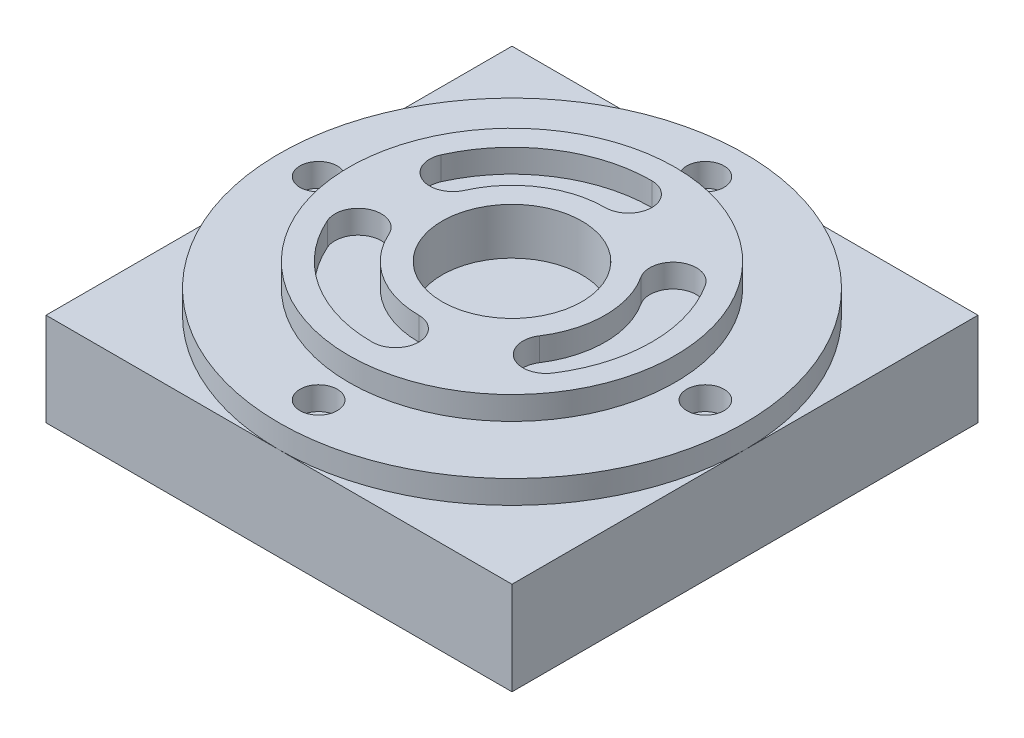
ISO-10303-21;
HEADER;
FILE_DESCRIPTION(('STEP AP214'),'2;1');
FILE_NAME('part.step','',(''),(''),'','','');
FILE_SCHEMA(('AUTOMOTIVE_DESIGN { 1 0 10303 214 1 1 1 1 }'));
ENDSEC;
DATA;
#1=APPLICATION_CONTEXT('core data for automotive mechanical design processes');
#2=APPLICATION_PROTOCOL_DEFINITION('international standard','automotive_design',2000,#1);
#3=PRODUCT_CONTEXT('',#1,'mechanical');
#4=PRODUCT('Part','Part','',(#3));
#5=PRODUCT_RELATED_PRODUCT_CATEGORY('part','',(#4));
#6=PRODUCT_DEFINITION_FORMATION('','',#4);
#7=PRODUCT_DEFINITION_CONTEXT('part definition',#1,'design');
#8=PRODUCT_DEFINITION('design','',#6,#7);
#9=PRODUCT_DEFINITION_SHAPE('','',#8);
#10=(LENGTH_UNIT() NAMED_UNIT(*) SI_UNIT(.MILLI.,.METRE.));
#11=(NAMED_UNIT(*) PLANE_ANGLE_UNIT() SI_UNIT($,.RADIAN.));
#12=(NAMED_UNIT(*) SI_UNIT($,.STERADIAN.) SOLID_ANGLE_UNIT());
#13=UNCERTAINTY_MEASURE_WITH_UNIT(LENGTH_MEASURE(1.E-05),#10,'distance_accuracy_value','');
#14=(GEOMETRIC_REPRESENTATION_CONTEXT(3) GLOBAL_UNCERTAINTY_ASSIGNED_CONTEXT((#13)) GLOBAL_UNIT_ASSIGNED_CONTEXT((#10,
#11,#12)) REPRESENTATION_CONTEXT('',''));
#15=CARTESIAN_POINT('',(0.,0.,0.));
#16=DIRECTION('',(0.,0.,1.));
#17=DIRECTION('',(1.,0.,0.));
#18=AXIS2_PLACEMENT_3D('',#15,#16,#17);
#19=CARTESIAN_POINT('',(0.,30.,0.));
#20=DIRECTION('',(0.,1.,0.));
#21=DIRECTION('',(0.,0.,1.));
#22=AXIS2_PLACEMENT_3D('',#19,#20,#21);
#23=PLANE('',#22);
#24=CARTESIAN_POINT('',(0.,30.,0.));
#25=DIRECTION('',(0.,1.,0.));
#26=DIRECTION('',(0.,0.,1.));
#27=AXIS2_PLACEMENT_3D('',#24,#25,#26);
#28=CIRCLE('',#27,15.);
#29=CARTESIAN_POINT('',(0.,30.,15.));
#30=VERTEX_POINT('',#29);
#31=EDGE_CURVE('E195',#30,#30,#28,.T.);
#32=ORIENTED_EDGE('',*,*,#31,.F.);
#33=EDGE_LOOP('',(#32));
#34=FACE_BOUND('',#33,.T.);
#35=CARTESIAN_POINT('',(0.,30.,0.));
#36=DIRECTION('',(0.,1.,0.));
#37=DIRECTION('',(0.,0.,1.));
#38=AXIS2_PLACEMENT_3D('',#35,#36,#37);
#39=CIRCLE('',#38,30.);
#40=CARTESIAN_POINT('',(0.,30.,-30.));
#41=VERTEX_POINT('',#40);
#42=CARTESIAN_POINT('',(-27.4052277606624,30.,-12.2046504));
#43=VERTEX_POINT('',#42);
#44=EDGE_CURVE('E62',#41,#43,#39,.T.);
#45=ORIENTED_EDGE('',*,*,#44,.F.);
#46=CARTESIAN_POINT('',(0.,30.,-25.));
#47=DIRECTION('',(0.,1.,0.));
#48=DIRECTION('',(0.,0.,-1.));
#49=AXIS2_PLACEMENT_3D('',#46,#47,#48);
#50=CIRCLE('',#49,5.);
#51=CARTESIAN_POINT('',(0.,30.,-20.));
#52=VERTEX_POINT('',#51);
#53=EDGE_CURVE('E213',#52,#41,#50,.T.);
#54=ORIENTED_EDGE('',*,*,#53,.F.);
#55=CARTESIAN_POINT('',(0.,30.,0.));
#56=DIRECTION('',(0.,-1.,0.));
#57=DIRECTION('',(0.,0.,1.));
#58=AXIS2_PLACEMENT_3D('',#55,#56,#57);
#59=CIRCLE('',#58,20.);
#60=CARTESIAN_POINT('',(-18.2701518404416,30.,-8.1364336));
#61=VERTEX_POINT('',#60);
#62=EDGE_CURVE('E230',#61,#52,#59,.T.);
#63=ORIENTED_EDGE('',*,*,#62,.F.);
#64=CARTESIAN_POINT('',(-22.837689800552,30.,-10.170542));
#65=DIRECTION('',(0.,1.,0.));
#66=DIRECTION('',(0.,0.,-1.));
#67=AXIS2_PLACEMENT_3D('',#64,#65,#66);
#68=CIRCLE('',#67,5.);
#69=EDGE_CURVE('E223',#43,#61,#68,.T.);
#70=ORIENTED_EDGE('',*,*,#69,.F.);
#71=EDGE_LOOP('',(#45,#54,#63,#70));
#72=FACE_BOUND('',#71,.T.);
#73=CARTESIAN_POINT('',(0.,30.,0.));
#74=DIRECTION('',(0.,1.,0.));
#75=DIRECTION('',(0.,0.,1.));
#76=AXIS2_PLACEMENT_3D('',#73,#74,#75);
#77=CIRCLE('',#76,35.);
#78=CARTESIAN_POINT('',(0.,30.,35.));
#79=VERTEX_POINT('',#78);
#80=EDGE_CURVE('E275',#79,#79,#77,.T.);
#81=ORIENTED_EDGE('',*,*,#80,.T.);
#82=EDGE_LOOP('',(#81));
#83=FACE_BOUND('',#82,.T.);
#84=CARTESIAN_POINT('',(0.,30.,25.));
#85=DIRECTION('',(0.,1.,0.));
#86=DIRECTION('',(0.,0.,-1.));
#87=AXIS2_PLACEMENT_3D('',#84,#85,#86);
#88=CIRCLE('',#87,5.);
#89=CARTESIAN_POINT('',(0.,30.,30.));
#90=VERTEX_POINT('',#89);
#91=CARTESIAN_POINT('',(0.,30.,20.));
#92=VERTEX_POINT('',#91);
#93=EDGE_CURVE('E251',#90,#92,#88,.T.);
#94=ORIENTED_EDGE('',*,*,#93,.F.);
#95=CARTESIAN_POINT('',(0.,30.,0.));
#96=DIRECTION('',(0.,1.,0.));
#97=DIRECTION('',(0.,0.,1.));
#98=AXIS2_PLACEMENT_3D('',#95,#96,#97);
#99=CIRCLE('',#98,30.);
#100=CARTESIAN_POINT('',(-27.4052277606624,30.,12.2046504));
#101=VERTEX_POINT('',#100);
#102=EDGE_CURVE('E242',#101,#90,#99,.T.);
#103=ORIENTED_EDGE('',*,*,#102,.F.);
#104=CARTESIAN_POINT('',(-22.837689800552,30.,10.170542));
#105=DIRECTION('',(0.,1.,0.));
#106=DIRECTION('',(0.,0.,1.));
#107=AXIS2_PLACEMENT_3D('',#104,#105,#106);
#108=CIRCLE('',#107,5.);
#109=CARTESIAN_POINT('',(-18.2701518404416,30.,8.13643360000001));
#110=VERTEX_POINT('',#109);
#111=EDGE_CURVE('E257',#110,#101,#108,.T.);
#112=ORIENTED_EDGE('',*,*,#111,.F.);
#113=CARTESIAN_POINT('',(0.,30.,0.));
#114=DIRECTION('',(0.,-1.,0.));
#115=DIRECTION('',(0.,0.,1.));
#116=AXIS2_PLACEMENT_3D('',#113,#114,#115);
#117=CIRCLE('',#116,20.);
#118=EDGE_CURVE('E259',#92,#110,#117,.T.);
#119=ORIENTED_EDGE('',*,*,#118,.F.);
#120=EDGE_LOOP('',(#94,#103,#112,#119));
#121=FACE_BOUND('',#120,.T.);
#122=CARTESIAN_POINT('',(0.,30.,0.));
#123=DIRECTION('',(0.,-1.,0.));
#124=DIRECTION('',(0.,0.,1.));
#125=AXIS2_PLACEMENT_3D('',#122,#123,#124);
#126=CIRCLE('',#125,20.);
#127=CARTESIAN_POINT('',(16.7734113589085,30.,-10.8927807003006));
#128=VERTEX_POINT('',#127);
#129=CARTESIAN_POINT('',(16.7734113589085,30.,10.8927807003006));
#130=VERTEX_POINT('',#129);
#131=EDGE_CURVE('E60',#128,#130,#126,.T.);
#132=ORIENTED_EDGE('',*,*,#131,.F.);
#133=CARTESIAN_POINT('',(20.9667641986356,30.,-13.6159758753757));
#134=DIRECTION('',(0.,1.,0.));
#135=DIRECTION('',(0.,0.,-1.));
#136=AXIS2_PLACEMENT_3D('',#133,#134,#135);
#137=CIRCLE('',#136,5.);
#138=CARTESIAN_POINT('',(25.1601170383627,30.,-16.3391710504508));
#139=VERTEX_POINT('',#138);
#140=EDGE_CURVE('E190',#139,#128,#137,.T.);
#141=ORIENTED_EDGE('',*,*,#140,.F.);
#142=CARTESIAN_POINT('',(0.,30.,0.));
#143=DIRECTION('',(0.,1.,0.));
#144=DIRECTION('',(0.,0.,1.));
#145=AXIS2_PLACEMENT_3D('',#142,#143,#144);
#146=CIRCLE('',#145,30.);
#147=CARTESIAN_POINT('',(25.1601170383627,30.,16.3391710504508));
#148=VERTEX_POINT('',#147);
#149=EDGE_CURVE('E188',#148,#139,#146,.T.);
#150=ORIENTED_EDGE('',*,*,#149,.F.);
#151=CARTESIAN_POINT('',(20.9667641986356,30.,13.6159758753757));
#152=DIRECTION('',(0.,1.,0.));
#153=DIRECTION('',(0.,0.,1.));
#154=AXIS2_PLACEMENT_3D('',#151,#152,#153);
#155=CIRCLE('',#154,5.);
#156=EDGE_CURVE('E199',#130,#148,#155,.T.);
#157=ORIENTED_EDGE('',*,*,#156,.F.);
#158=EDGE_LOOP('',(#132,#141,#150,#157));
#159=FACE_BOUND('',#158,.T.);
#160=ADVANCED_FACE('F39',(#34,#72,#83,#121,#159),#23,.T.);
#161=CARTESIAN_POINT('',(0.,20.,0.));
#162=DIRECTION('',(0.,1.,0.));
#163=DIRECTION('',(0.,0.,1.));
#164=AXIS2_PLACEMENT_3D('',#161,#162,#163);
#165=PLANE('',#164);
#166=CARTESIAN_POINT('',(0.,20.,0.));
#167=DIRECTION('',(0.,1.,0.));
#168=DIRECTION('',(0.,0.,1.));
#169=AXIS2_PLACEMENT_3D('',#166,#167,#168);
#170=CIRCLE('',#169,50.);
#171=CARTESIAN_POINT('',(0.,20.,50.));
#172=VERTEX_POINT('',#171);
#173=CARTESIAN_POINT('',(50.,20.,0.));
#174=VERTEX_POINT('',#173);
#175=EDGE_CURVE('E49',#172,#174,#170,.T.);
#176=ORIENTED_EDGE('',*,*,#175,.F.);
#177=DIRECTION('',(1.,0.,0.));
#178=VECTOR('',#177,1.);
#179=CARTESIAN_POINT('',(-50.,20.,50.));
#180=LINE('',#179,#178);
#181=CARTESIAN_POINT('',(50.,20.,50.));
#182=VERTEX_POINT('',#181);
#183=EDGE_CURVE('E316',#172,#182,#180,.T.);
#184=ORIENTED_EDGE('',*,*,#183,.T.);
#185=DIRECTION('',(0.,0.,-1.));
#186=VECTOR('',#185,1.);
#187=CARTESIAN_POINT('',(50.,20.,-50.));
#188=LINE('',#187,#186);
#189=EDGE_CURVE('E310',#182,#174,#188,.T.);
#190=ORIENTED_EDGE('',*,*,#189,.T.);
#191=EDGE_LOOP('',(#176,#184,#190));
#192=FACE_BOUND('',#191,.T.);
#193=ADVANCED_FACE('F359',(#192),#165,.T.);
#194=CARTESIAN_POINT('',(0.,20.,-50.));
#195=VERTEX_POINT('',#194);
#196=EDGE_CURVE('E11',#174,#195,#170,.T.);
#197=ORIENTED_EDGE('',*,*,#196,.F.);
#198=CARTESIAN_POINT('',(50.,20.,-50.));
#199=VERTEX_POINT('',#198);
#200=EDGE_CURVE('E311',#174,#199,#188,.T.);
#201=ORIENTED_EDGE('',*,*,#200,.T.);
#202=DIRECTION('',(-1.,0.,0.));
#203=VECTOR('',#202,1.);
#204=CARTESIAN_POINT('',(-50.,20.,-50.));
#205=LINE('',#204,#203);
#206=EDGE_CURVE('E315',#199,#195,#205,.T.);
#207=ORIENTED_EDGE('',*,*,#206,.T.);
#208=EDGE_LOOP('',(#197,#201,#207));
#209=FACE_BOUND('',#208,.T.);
#210=ADVANCED_FACE('F351',(#209),#165,.T.);
#211=CARTESIAN_POINT('',(-50.,20.,0.));
#212=VERTEX_POINT('',#211);
#213=EDGE_CURVE('E48',#195,#212,#170,.T.);
#214=ORIENTED_EDGE('',*,*,#213,.F.);
#215=CARTESIAN_POINT('',(-50.,20.,-50.));
#216=VERTEX_POINT('',#215);
#217=EDGE_CURVE('E309',#195,#216,#205,.T.);
#218=ORIENTED_EDGE('',*,*,#217,.T.);
#219=DIRECTION('',(0.,0.,1.));
#220=VECTOR('',#219,1.);
#221=CARTESIAN_POINT('',(-50.,20.,-50.));
#222=LINE('',#221,#220);
#223=EDGE_CURVE('E317',#216,#212,#222,.T.);
#224=ORIENTED_EDGE('',*,*,#223,.T.);
#225=EDGE_LOOP('',(#214,#218,#224));
#226=FACE_BOUND('',#225,.T.);
#227=ADVANCED_FACE('F352',(#226),#165,.T.);
#228=CARTESIAN_POINT('',(50.,20.,-50.));
#229=DIRECTION('',(-1.,0.,0.));
#230=DIRECTION('',(0.,0.,1.));
#231=AXIS2_PLACEMENT_3D('',#228,#229,#230);
#232=PLANE('',#231);
#233=DIRECTION('',(0.,0.,-1.));
#234=VECTOR('',#233,1.);
#235=CARTESIAN_POINT('',(50.,0.,-50.));
#236=LINE('',#235,#234);
#237=CARTESIAN_POINT('',(50.,0.,50.));
#238=VERTEX_POINT('',#237);
#239=CARTESIAN_POINT('',(50.,0.,-50.));
#240=VERTEX_POINT('',#239);
#241=EDGE_CURVE('E303',#238,#240,#236,.T.);
#242=ORIENTED_EDGE('',*,*,#241,.T.);
#243=DIRECTION('',(0.,-1.,0.));
#244=VECTOR('',#243,1.);
#245=CARTESIAN_POINT('',(50.,20.,-50.));
#246=LINE('',#245,#244);
#247=EDGE_CURVE('E43',#199,#240,#246,.T.);
#248=ORIENTED_EDGE('',*,*,#247,.F.);
#249=ORIENTED_EDGE('',*,*,#200,.F.);
#250=ORIENTED_EDGE('',*,*,#189,.F.);
#251=DIRECTION('',(0.,-1.,0.));
#252=VECTOR('',#251,1.);
#253=CARTESIAN_POINT('',(50.,20.,50.));
#254=LINE('',#253,#252);
#255=EDGE_CURVE('E321',#182,#238,#254,.T.);
#256=ORIENTED_EDGE('',*,*,#255,.T.);
#257=EDGE_LOOP('',(#242,#248,#249,#250,#256));
#258=FACE_BOUND('',#257,.T.);
#259=ADVANCED_FACE('F41',(#258),#232,.F.);
#260=CARTESIAN_POINT('',(-50.,20.,-50.));
#261=DIRECTION('',(0.,0.,1.));
#262=DIRECTION('',(1.,0.,0.));
#263=AXIS2_PLACEMENT_3D('',#260,#261,#262);
#264=PLANE('',#263);
#265=DIRECTION('',(-1.,0.,0.));
#266=VECTOR('',#265,1.);
#267=CARTESIAN_POINT('',(-50.,0.,-50.));
#268=LINE('',#267,#266);
#269=CARTESIAN_POINT('',(-50.,0.,-50.));
#270=VERTEX_POINT('',#269);
#271=EDGE_CURVE('E322',#240,#270,#268,.T.);
#272=ORIENTED_EDGE('',*,*,#271,.T.);
#273=DIRECTION('',(0.,-1.,0.));
#274=VECTOR('',#273,1.);
#275=CARTESIAN_POINT('',(-50.,20.,-50.));
#276=LINE('',#275,#274);
#277=EDGE_CURVE('E333',#216,#270,#276,.T.);
#278=ORIENTED_EDGE('',*,*,#277,.F.);
#279=ORIENTED_EDGE('',*,*,#217,.F.);
#280=ORIENTED_EDGE('',*,*,#206,.F.);
#281=ORIENTED_EDGE('',*,*,#247,.T.);
#282=EDGE_LOOP('',(#272,#278,#279,#280,#281));
#283=FACE_BOUND('',#282,.T.);
#284=ADVANCED_FACE('F354',(#283),#264,.F.);
#285=CARTESIAN_POINT('',(-50.,20.,-50.));
#286=DIRECTION('',(1.,0.,0.));
#287=DIRECTION('',(0.,0.,-1.));
#288=AXIS2_PLACEMENT_3D('',#285,#286,#287);
#289=PLANE('',#288);
#290=DIRECTION('',(0.,0.,1.));
#291=VECTOR('',#290,1.);
#292=CARTESIAN_POINT('',(-50.,0.,-50.));
#293=LINE('',#292,#291);
#294=CARTESIAN_POINT('',(-50.,0.,50.));
#295=VERTEX_POINT('',#294);
#296=EDGE_CURVE('E330',#270,#295,#293,.T.);
#297=ORIENTED_EDGE('',*,*,#296,.T.);
#298=DIRECTION('',(0.,-1.,0.));
#299=VECTOR('',#298,1.);
#300=CARTESIAN_POINT('',(-50.,20.,50.));
#301=LINE('',#300,#299);
#302=CARTESIAN_POINT('',(-50.,20.,50.));
#303=VERTEX_POINT('',#302);
#304=EDGE_CURVE('E335',#303,#295,#301,.T.);
#305=ORIENTED_EDGE('',*,*,#304,.F.);
#306=EDGE_CURVE('E314',#212,#303,#222,.T.);
#307=ORIENTED_EDGE('',*,*,#306,.F.);
#308=ORIENTED_EDGE('',*,*,#223,.F.);
#309=ORIENTED_EDGE('',*,*,#277,.T.);
#310=EDGE_LOOP('',(#297,#305,#307,#308,#309));
#311=FACE_BOUND('',#310,.T.);
#312=ADVANCED_FACE('F371',(#311),#289,.F.);
#313=CARTESIAN_POINT('',(-50.,20.,50.));
#314=DIRECTION('',(0.,0.,-1.));
#315=DIRECTION('',(-1.,0.,0.));
#316=AXIS2_PLACEMENT_3D('',#313,#314,#315);
#317=PLANE('',#316);
#318=DIRECTION('',(1.,0.,0.));
#319=VECTOR('',#318,1.);
#320=CARTESIAN_POINT('',(-50.,0.,50.));
#321=LINE('',#320,#319);
#322=EDGE_CURVE('E329',#295,#238,#321,.T.);
#323=ORIENTED_EDGE('',*,*,#322,.T.);
#324=ORIENTED_EDGE('',*,*,#255,.F.);
#325=ORIENTED_EDGE('',*,*,#183,.F.);
#326=EDGE_CURVE('E318',#303,#172,#180,.T.);
#327=ORIENTED_EDGE('',*,*,#326,.F.);
#328=ORIENTED_EDGE('',*,*,#304,.T.);
#329=EDGE_LOOP('',(#323,#324,#325,#327,#328));
#330=FACE_BOUND('',#329,.T.);
#331=ADVANCED_FACE('F362',(#330),#317,.F.);
#332=EDGE_CURVE('E306',#212,#172,#170,.T.);
#333=ORIENTED_EDGE('',*,*,#332,.F.);
#334=ORIENTED_EDGE('',*,*,#306,.T.);
#335=ORIENTED_EDGE('',*,*,#326,.T.);
#336=EDGE_LOOP('',(#333,#334,#335));
#337=FACE_BOUND('',#336,.T.);
#338=ADVANCED_FACE('F372',(#337),#165,.T.);
#339=CARTESIAN_POINT('',(0.,0.,0.));
#340=DIRECTION('',(0.,1.,0.));
#341=DIRECTION('',(0.,0.,1.));
#342=AXIS2_PLACEMENT_3D('',#339,#340,#341);
#343=PLANE('',#342);
#344=ORIENTED_EDGE('',*,*,#241,.F.);
#345=ORIENTED_EDGE('',*,*,#322,.F.);
#346=ORIENTED_EDGE('',*,*,#296,.F.);
#347=ORIENTED_EDGE('',*,*,#271,.F.);
#348=EDGE_LOOP('',(#344,#345,#346,#347));
#349=FACE_BOUND('',#348,.T.);
#350=ADVANCED_FACE('F367',(#349),#343,.F.);
#351=CARTESIAN_POINT('',(0.,25.,0.));
#352=DIRECTION('',(0.,-1.,0.));
#353=DIRECTION('',(0.,0.,-1.));
#354=AXIS2_PLACEMENT_3D('',#351,#352,#353);
#355=CYLINDRICAL_SURFACE('',#354,50.);
#356=CARTESIAN_POINT('',(0.,25.,0.));
#357=DIRECTION('',(0.,1.,0.));
#358=DIRECTION('',(0.,0.,1.));
#359=AXIS2_PLACEMENT_3D('',#356,#357,#358);
#360=CIRCLE('',#359,50.);
#361=CARTESIAN_POINT('',(0.,25.,50.));
#362=VERTEX_POINT('',#361);
#363=EDGE_CURVE('E301',#362,#362,#360,.T.);
#364=ORIENTED_EDGE('',*,*,#363,.F.);
#365=EDGE_LOOP('',(#364));
#366=FACE_BOUND('',#365,.T.);
#367=ORIENTED_EDGE('',*,*,#175,.T.);
#368=ORIENTED_EDGE('',*,*,#196,.T.);
#369=ORIENTED_EDGE('',*,*,#213,.T.);
#370=ORIENTED_EDGE('',*,*,#332,.T.);
#371=EDGE_LOOP('',(#367,#368,#369,#370));
#372=FACE_BOUND('',#371,.T.);
#373=ADVANCED_FACE('F346',(#366,#372),#355,.T.);
#374=CARTESIAN_POINT('',(0.,25.,0.));
#375=DIRECTION('',(0.,1.,0.));
#376=DIRECTION('',(0.,0.,1.));
#377=AXIS2_PLACEMENT_3D('',#374,#375,#376);
#378=PLANE('',#377);
#379=CARTESIAN_POINT('',(0.,25.,0.));
#380=DIRECTION('',(0.,1.,0.));
#381=DIRECTION('',(0.,0.,1.));
#382=AXIS2_PLACEMENT_3D('',#379,#380,#381);
#383=CIRCLE('',#382,35.);
#384=CARTESIAN_POINT('',(0.,25.,35.));
#385=VERTEX_POINT('',#384);
#386=EDGE_CURVE('E207',#385,#385,#383,.T.);
#387=ORIENTED_EDGE('',*,*,#386,.F.);
#388=EDGE_LOOP('',(#387));
#389=FACE_BOUND('',#388,.T.);
#390=CARTESIAN_POINT('',(0.,25.,-41.5));
#391=DIRECTION('',(0.,1.,0.));
#392=DIRECTION('',(0.,0.,1.));
#393=AXIS2_PLACEMENT_3D('',#390,#391,#392);
#394=CIRCLE('',#393,4.);
#395=CARTESIAN_POINT('',(0.,25.,-37.5));
#396=VERTEX_POINT('',#395);
#397=EDGE_CURVE('E283',#396,#396,#394,.T.);
#398=ORIENTED_EDGE('',*,*,#397,.F.);
#399=EDGE_LOOP('',(#398));
#400=FACE_BOUND('',#399,.T.);
#401=CARTESIAN_POINT('',(41.5,25.,0.));
#402=DIRECTION('',(0.,1.,0.));
#403=DIRECTION('',(0.,0.,1.));
#404=AXIS2_PLACEMENT_3D('',#401,#402,#403);
#405=CIRCLE('',#404,4.);
#406=CARTESIAN_POINT('',(41.5,25.,4.));
#407=VERTEX_POINT('',#406);
#408=EDGE_CURVE('E289',#407,#407,#405,.T.);
#409=ORIENTED_EDGE('',*,*,#408,.F.);
#410=EDGE_LOOP('',(#409));
#411=FACE_BOUND('',#410,.T.);
#412=CARTESIAN_POINT('',(0.,25.,41.5));
#413=DIRECTION('',(0.,1.,0.));
#414=DIRECTION('',(0.,0.,1.));
#415=AXIS2_PLACEMENT_3D('',#412,#413,#414);
#416=CIRCLE('',#415,4.);
#417=CARTESIAN_POINT('',(0.,25.,45.5));
#418=VERTEX_POINT('',#417);
#419=EDGE_CURVE('E291',#418,#418,#416,.T.);
#420=ORIENTED_EDGE('',*,*,#419,.F.);
#421=EDGE_LOOP('',(#420));
#422=FACE_BOUND('',#421,.T.);
#423=CARTESIAN_POINT('',(-41.5,25.,0.));
#424=DIRECTION('',(0.,1.,0.));
#425=DIRECTION('',(0.,0.,1.));
#426=AXIS2_PLACEMENT_3D('',#423,#424,#425);
#427=CIRCLE('',#426,4.);
#428=CARTESIAN_POINT('',(-41.5,25.,4.));
#429=VERTEX_POINT('',#428);
#430=EDGE_CURVE('E273',#429,#429,#427,.T.);
#431=ORIENTED_EDGE('',*,*,#430,.F.);
#432=EDGE_LOOP('',(#431));
#433=FACE_BOUND('',#432,.T.);
#434=ORIENTED_EDGE('',*,*,#363,.T.);
#435=EDGE_LOOP('',(#434));
#436=FACE_BOUND('',#435,.T.);
#437=ADVANCED_FACE('F434',(#389,#400,#411,#422,#433,#436),#378,.T.);
#438=CARTESIAN_POINT('',(-41.5,20.,0.));
#439=DIRECTION('',(0.,1.,0.));
#440=DIRECTION('',(0.,0.,1.));
#441=AXIS2_PLACEMENT_3D('',#438,#439,#440);
#442=CYLINDRICAL_SURFACE('',#441,4.);
#443=CARTESIAN_POINT('',(-41.5,20.,0.));
#444=DIRECTION('',(0.,1.,0.));
#445=DIRECTION('',(0.,0.,1.));
#446=AXIS2_PLACEMENT_3D('',#443,#444,#445);
#447=CIRCLE('',#446,4.);
#448=CARTESIAN_POINT('',(-41.5,20.,4.));
#449=VERTEX_POINT('',#448);
#450=EDGE_CURVE('E298',#449,#449,#447,.T.);
#451=ORIENTED_EDGE('',*,*,#450,.F.);
#452=EDGE_LOOP('',(#451));
#453=FACE_BOUND('',#452,.T.);
#454=ORIENTED_EDGE('',*,*,#430,.T.);
#455=EDGE_LOOP('',(#454));
#456=FACE_BOUND('',#455,.T.);
#457=ADVANCED_FACE('F431',(#453,#456),#442,.F.);
#458=CARTESIAN_POINT('',(-41.5,20.,0.));
#459=DIRECTION('',(0.,1.,0.));
#460=DIRECTION('',(0.,0.,1.));
#461=AXIS2_PLACEMENT_3D('',#458,#459,#460);
#462=PLANE('',#461);
#463=ORIENTED_EDGE('',*,*,#450,.T.);
#464=EDGE_LOOP('',(#463));
#465=FACE_BOUND('',#464,.T.);
#466=ADVANCED_FACE('F430',(#465),#462,.T.);
#467=CARTESIAN_POINT('',(0.,20.,41.5));
#468=DIRECTION('',(0.,1.,0.));
#469=DIRECTION('',(0.,0.,1.));
#470=AXIS2_PLACEMENT_3D('',#467,#468,#469);
#471=CYLINDRICAL_SURFACE('',#470,4.);
#472=CARTESIAN_POINT('',(0.,20.,41.5));
#473=DIRECTION('',(0.,1.,0.));
#474=DIRECTION('',(0.,0.,1.));
#475=AXIS2_PLACEMENT_3D('',#472,#473,#474);
#476=CIRCLE('',#475,4.);
#477=CARTESIAN_POINT('',(0.,20.,45.5));
#478=VERTEX_POINT('',#477);
#479=EDGE_CURVE('E288',#478,#478,#476,.T.);
#480=ORIENTED_EDGE('',*,*,#479,.F.);
#481=EDGE_LOOP('',(#480));
#482=FACE_BOUND('',#481,.T.);
#483=ORIENTED_EDGE('',*,*,#419,.T.);
#484=EDGE_LOOP('',(#483));
#485=FACE_BOUND('',#484,.T.);
#486=ADVANCED_FACE('F421',(#482,#485),#471,.F.);
#487=CARTESIAN_POINT('',(0.,20.,41.5));
#488=DIRECTION('',(0.,1.,0.));
#489=DIRECTION('',(0.,0.,1.));
#490=AXIS2_PLACEMENT_3D('',#487,#488,#489);
#491=PLANE('',#490);
#492=ORIENTED_EDGE('',*,*,#479,.T.);
#493=EDGE_LOOP('',(#492));
#494=FACE_BOUND('',#493,.T.);
#495=ADVANCED_FACE('F416',(#494),#491,.T.);
#496=CARTESIAN_POINT('',(41.5,20.,0.));
#497=DIRECTION('',(0.,1.,0.));
#498=DIRECTION('',(0.,0.,1.));
#499=AXIS2_PLACEMENT_3D('',#496,#497,#498);
#500=CYLINDRICAL_SURFACE('',#499,4.);
#501=CARTESIAN_POINT('',(41.5,20.,0.));
#502=DIRECTION('',(0.,1.,0.));
#503=DIRECTION('',(0.,0.,1.));
#504=AXIS2_PLACEMENT_3D('',#501,#502,#503);
#505=CIRCLE('',#504,4.);
#506=CARTESIAN_POINT('',(41.5,20.,4.));
#507=VERTEX_POINT('',#506);
#508=EDGE_CURVE('E284',#507,#507,#505,.T.);
#509=ORIENTED_EDGE('',*,*,#508,.F.);
#510=EDGE_LOOP('',(#509));
#511=FACE_BOUND('',#510,.T.);
#512=ORIENTED_EDGE('',*,*,#408,.T.);
#513=EDGE_LOOP('',(#512));
#514=FACE_BOUND('',#513,.T.);
#515=ADVANCED_FACE('F412',(#511,#514),#500,.F.);
#516=CARTESIAN_POINT('',(41.5,20.,0.));
#517=DIRECTION('',(0.,1.,0.));
#518=DIRECTION('',(0.,0.,1.));
#519=AXIS2_PLACEMENT_3D('',#516,#517,#518);
#520=PLANE('',#519);
#521=ORIENTED_EDGE('',*,*,#508,.T.);
#522=EDGE_LOOP('',(#521));
#523=FACE_BOUND('',#522,.T.);
#524=ADVANCED_FACE('F413',(#523),#520,.T.);
#525=CARTESIAN_POINT('',(0.,20.,-41.5));
#526=DIRECTION('',(0.,1.,0.));
#527=DIRECTION('',(0.,0.,1.));
#528=AXIS2_PLACEMENT_3D('',#525,#526,#527);
#529=CYLINDRICAL_SURFACE('',#528,4.);
#530=CARTESIAN_POINT('',(0.,20.,-41.5));
#531=DIRECTION('',(0.,1.,0.));
#532=DIRECTION('',(0.,0.,1.));
#533=AXIS2_PLACEMENT_3D('',#530,#531,#532);
#534=CIRCLE('',#533,4.);
#535=CARTESIAN_POINT('',(0.,20.,-37.5));
#536=VERTEX_POINT('',#535);
#537=EDGE_CURVE('E280',#536,#536,#534,.T.);
#538=ORIENTED_EDGE('',*,*,#537,.F.);
#539=EDGE_LOOP('',(#538));
#540=FACE_BOUND('',#539,.T.);
#541=ORIENTED_EDGE('',*,*,#397,.T.);
#542=EDGE_LOOP('',(#541));
#543=FACE_BOUND('',#542,.T.);
#544=ADVANCED_FACE('F406',(#540,#543),#529,.F.);
#545=CARTESIAN_POINT('',(0.,20.,-41.5));
#546=DIRECTION('',(0.,1.,0.));
#547=DIRECTION('',(0.,0.,1.));
#548=AXIS2_PLACEMENT_3D('',#545,#546,#547);
#549=PLANE('',#548);
#550=ORIENTED_EDGE('',*,*,#537,.T.);
#551=EDGE_LOOP('',(#550));
#552=FACE_BOUND('',#551,.T.);
#553=ADVANCED_FACE('F401',(#552),#549,.T.);
#554=CARTESIAN_POINT('',(0.,30.,0.));
#555=DIRECTION('',(0.,-1.,0.));
#556=DIRECTION('',(0.,0.,-1.));
#557=AXIS2_PLACEMENT_3D('',#554,#555,#556);
#558=CYLINDRICAL_SURFACE('',#557,35.);
#559=ORIENTED_EDGE('',*,*,#80,.F.);
#560=EDGE_LOOP('',(#559));
#561=FACE_BOUND('',#560,.T.);
#562=ORIENTED_EDGE('',*,*,#386,.T.);
#563=EDGE_LOOP('',(#562));
#564=FACE_BOUND('',#563,.T.);
#565=ADVANCED_FACE('F398',(#561,#564),#558,.T.);
#566=CARTESIAN_POINT('',(0.,25.,25.));
#567=DIRECTION('',(0.,1.,0.));
#568=DIRECTION('',(0.,0.,1.));
#569=AXIS2_PLACEMENT_3D('',#566,#567,#568);
#570=CYLINDRICAL_SURFACE('',#569,5.);
#571=ORIENTED_EDGE('',*,*,#93,.T.);
#572=DIRECTION('',(0.,1.,0.));
#573=VECTOR('',#572,1.);
#574=CARTESIAN_POINT('',(0.,25.,20.));
#575=LINE('',#574,#573);
#576=CARTESIAN_POINT('',(0.,25.,20.));
#577=VERTEX_POINT('',#576);
#578=EDGE_CURVE('E254',#577,#92,#575,.T.);
#579=ORIENTED_EDGE('',*,*,#578,.F.);
#580=CARTESIAN_POINT('',(0.,25.,25.));
#581=DIRECTION('',(0.,1.,0.));
#582=DIRECTION('',(0.,0.,-1.));
#583=AXIS2_PLACEMENT_3D('',#580,#581,#582);
#584=CIRCLE('',#583,5.);
#585=CARTESIAN_POINT('',(0.,25.,30.));
#586=VERTEX_POINT('',#585);
#587=EDGE_CURVE('E239',#586,#577,#584,.T.);
#588=ORIENTED_EDGE('',*,*,#587,.F.);
#589=DIRECTION('',(0.,1.,0.));
#590=VECTOR('',#589,1.);
#591=CARTESIAN_POINT('',(0.,25.,30.));
#592=LINE('',#591,#590);
#593=EDGE_CURVE('E228',#586,#90,#592,.T.);
#594=ORIENTED_EDGE('',*,*,#593,.T.);
#595=EDGE_LOOP('',(#571,#579,#588,#594));
#596=FACE_BOUND('',#595,.T.);
#597=ADVANCED_FACE('F400',(#596),#570,.F.);
#598=CARTESIAN_POINT('',(0.,25.,0.));
#599=DIRECTION('',(0.,1.,0.));
#600=DIRECTION('',(0.,0.,1.));
#601=AXIS2_PLACEMENT_3D('',#598,#599,#600);
#602=CYLINDRICAL_SURFACE('',#601,30.);
#603=ORIENTED_EDGE('',*,*,#102,.T.);
#604=ORIENTED_EDGE('',*,*,#593,.F.);
#605=CARTESIAN_POINT('',(0.,25.,0.));
#606=DIRECTION('',(0.,1.,0.));
#607=DIRECTION('',(0.,0.,1.));
#608=AXIS2_PLACEMENT_3D('',#605,#606,#607);
#609=CIRCLE('',#608,30.);
#610=CARTESIAN_POINT('',(-27.4052277606624,25.,12.2046504));
#611=VERTEX_POINT('',#610);
#612=EDGE_CURVE('E249',#611,#586,#609,.T.);
#613=ORIENTED_EDGE('',*,*,#612,.F.);
#614=DIRECTION('',(0.,1.,0.));
#615=VECTOR('',#614,1.);
#616=CARTESIAN_POINT('',(-27.4052277606624,25.,12.2046504));
#617=LINE('',#616,#615);
#618=EDGE_CURVE('E267',#611,#101,#617,.T.);
#619=ORIENTED_EDGE('',*,*,#618,.T.);
#620=EDGE_LOOP('',(#603,#604,#613,#619));
#621=FACE_BOUND('',#620,.T.);
#622=ADVANCED_FACE('F503',(#621),#602,.F.);
#623=CARTESIAN_POINT('',(-22.837689800552,25.,10.170542));
#624=DIRECTION('',(0.,1.,0.));
#625=DIRECTION('',(0.,0.,1.));
#626=AXIS2_PLACEMENT_3D('',#623,#624,#625);
#627=CYLINDRICAL_SURFACE('',#626,5.);
#628=ORIENTED_EDGE('',*,*,#111,.T.);
#629=ORIENTED_EDGE('',*,*,#618,.F.);
#630=CARTESIAN_POINT('',(-22.837689800552,25.,10.170542));
#631=DIRECTION('',(0.,1.,0.));
#632=DIRECTION('',(0.,0.,1.));
#633=AXIS2_PLACEMENT_3D('',#630,#631,#632);
#634=CIRCLE('',#633,5.);
#635=CARTESIAN_POINT('',(-18.2701518404416,25.,8.13643360000001));
#636=VERTEX_POINT('',#635);
#637=EDGE_CURVE('E250',#636,#611,#634,.T.);
#638=ORIENTED_EDGE('',*,*,#637,.F.);
#639=DIRECTION('',(0.,1.,0.));
#640=VECTOR('',#639,1.);
#641=CARTESIAN_POINT('',(-18.2701518404416,25.,8.13643360000001));
#642=LINE('',#641,#640);
#643=EDGE_CURVE('E270',#636,#110,#642,.T.);
#644=ORIENTED_EDGE('',*,*,#643,.T.);
#645=EDGE_LOOP('',(#628,#629,#638,#644));
#646=FACE_BOUND('',#645,.T.);
#647=ADVANCED_FACE('F512',(#646),#627,.F.);
#648=CARTESIAN_POINT('',(0.,25.,0.));
#649=DIRECTION('',(0.,1.,0.));
#650=DIRECTION('',(0.,0.,1.));
#651=AXIS2_PLACEMENT_3D('',#648,#649,#650);
#652=CYLINDRICAL_SURFACE('',#651,20.);
#653=ORIENTED_EDGE('',*,*,#118,.T.);
#654=ORIENTED_EDGE('',*,*,#643,.F.);
#655=CARTESIAN_POINT('',(0.,25.,0.));
#656=DIRECTION('',(0.,-1.,0.));
#657=DIRECTION('',(0.,0.,1.));
#658=AXIS2_PLACEMENT_3D('',#655,#656,#657);
#659=CIRCLE('',#658,20.);
#660=EDGE_CURVE('E243',#577,#636,#659,.T.);
#661=ORIENTED_EDGE('',*,*,#660,.F.);
#662=ORIENTED_EDGE('',*,*,#578,.T.);
#663=EDGE_LOOP('',(#653,#654,#661,#662));
#664=FACE_BOUND('',#663,.T.);
#665=ADVANCED_FACE('F517',(#664),#652,.T.);
#666=CARTESIAN_POINT('',(0.,25.,12.5));
#667=DIRECTION('',(0.,-1.,0.));
#668=DIRECTION('',(0.,0.,-1.));
#669=AXIS2_PLACEMENT_3D('',#666,#667,#668);
#670=PLANE('',#669);
#671=ORIENTED_EDGE('',*,*,#587,.T.);
#672=ORIENTED_EDGE('',*,*,#660,.T.);
#673=ORIENTED_EDGE('',*,*,#637,.T.);
#674=ORIENTED_EDGE('',*,*,#612,.T.);
#675=EDGE_LOOP('',(#671,#672,#673,#674));
#676=FACE_BOUND('',#675,.T.);
#677=ADVANCED_FACE('F526',(#676),#670,.F.);
#678=CARTESIAN_POINT('',(0.,25.,0.));
#679=DIRECTION('',(0.,1.,0.));
#680=DIRECTION('',(0.,0.,1.));
#681=AXIS2_PLACEMENT_3D('',#678,#679,#680);
#682=CYLINDRICAL_SURFACE('',#681,30.);
#683=ORIENTED_EDGE('',*,*,#44,.T.);
#684=DIRECTION('',(0.,1.,0.));
#685=VECTOR('',#684,1.);
#686=CARTESIAN_POINT('',(-27.4052277606624,25.,-12.2046504));
#687=LINE('',#686,#685);
#688=CARTESIAN_POINT('',(-27.4052277606624,25.,-12.2046504));
#689=VERTEX_POINT('',#688);
#690=EDGE_CURVE('E225',#689,#43,#687,.T.);
#691=ORIENTED_EDGE('',*,*,#690,.F.);
#692=CARTESIAN_POINT('',(0.,25.,0.));
#693=DIRECTION('',(0.,1.,0.));
#694=DIRECTION('',(0.,0.,1.));
#695=AXIS2_PLACEMENT_3D('',#692,#693,#694);
#696=CIRCLE('',#695,30.);
#697=CARTESIAN_POINT('',(0.,25.,-30.));
#698=VERTEX_POINT('',#697);
#699=EDGE_CURVE('E208',#698,#689,#696,.T.);
#700=ORIENTED_EDGE('',*,*,#699,.F.);
#701=DIRECTION('',(0.,1.,0.));
#702=VECTOR('',#701,1.);
#703=CARTESIAN_POINT('',(0.,25.,-30.));
#704=LINE('',#703,#702);
#705=EDGE_CURVE('E197',#698,#41,#704,.T.);
#706=ORIENTED_EDGE('',*,*,#705,.T.);
#707=EDGE_LOOP('',(#683,#691,#700,#706));
#708=FACE_BOUND('',#707,.T.);
#709=ADVANCED_FACE('F536',(#708),#682,.F.);
#710=CARTESIAN_POINT('',(0.,25.,-25.));
#711=DIRECTION('',(0.,1.,0.));
#712=DIRECTION('',(0.,0.,1.));
#713=AXIS2_PLACEMENT_3D('',#710,#711,#712);
#714=CYLINDRICAL_SURFACE('',#713,5.);
#715=ORIENTED_EDGE('',*,*,#53,.T.);
#716=ORIENTED_EDGE('',*,*,#705,.F.);
#717=CARTESIAN_POINT('',(0.,25.,-25.));
#718=DIRECTION('',(0.,1.,0.));
#719=DIRECTION('',(0.,0.,-1.));
#720=AXIS2_PLACEMENT_3D('',#717,#718,#719);
#721=CIRCLE('',#720,5.);
#722=CARTESIAN_POINT('',(0.,25.,-20.));
#723=VERTEX_POINT('',#722);
#724=EDGE_CURVE('E217',#723,#698,#721,.T.);
#725=ORIENTED_EDGE('',*,*,#724,.F.);
#726=DIRECTION('',(0.,1.,0.));
#727=VECTOR('',#726,1.);
#728=CARTESIAN_POINT('',(0.,25.,-20.));
#729=LINE('',#728,#727);
#730=EDGE_CURVE('E232',#723,#52,#729,.T.);
#731=ORIENTED_EDGE('',*,*,#730,.T.);
#732=EDGE_LOOP('',(#715,#716,#725,#731));
#733=FACE_BOUND('',#732,.T.);
#734=ADVANCED_FACE('F547',(#733),#714,.F.);
#735=CARTESIAN_POINT('',(0.,25.,0.));
#736=DIRECTION('',(0.,1.,0.));
#737=DIRECTION('',(0.,0.,1.));
#738=AXIS2_PLACEMENT_3D('',#735,#736,#737);
#739=CYLINDRICAL_SURFACE('',#738,20.);
#740=ORIENTED_EDGE('',*,*,#62,.T.);
#741=ORIENTED_EDGE('',*,*,#730,.F.);
#742=CARTESIAN_POINT('',(0.,25.,0.));
#743=DIRECTION('',(0.,-1.,0.));
#744=DIRECTION('',(0.,0.,1.));
#745=AXIS2_PLACEMENT_3D('',#742,#743,#744);
#746=CIRCLE('',#745,20.);
#747=CARTESIAN_POINT('',(-18.2701518404416,25.,-8.1364336));
#748=VERTEX_POINT('',#747);
#749=EDGE_CURVE('E220',#748,#723,#746,.T.);
#750=ORIENTED_EDGE('',*,*,#749,.F.);
#751=DIRECTION('',(0.,1.,0.));
#752=VECTOR('',#751,1.);
#753=CARTESIAN_POINT('',(-18.2701518404416,25.,-8.1364336));
#754=LINE('',#753,#752);
#755=EDGE_CURVE('E240',#748,#61,#754,.T.);
#756=ORIENTED_EDGE('',*,*,#755,.T.);
#757=EDGE_LOOP('',(#740,#741,#750,#756));
#758=FACE_BOUND('',#757,.T.);
#759=ADVANCED_FACE('F555',(#758),#739,.T.);
#760=CARTESIAN_POINT('',(-22.837689800552,25.,-10.170542));
#761=DIRECTION('',(0.,1.,0.));
#762=DIRECTION('',(0.,0.,1.));
#763=AXIS2_PLACEMENT_3D('',#760,#761,#762);
#764=CYLINDRICAL_SURFACE('',#763,5.);
#765=ORIENTED_EDGE('',*,*,#69,.T.);
#766=ORIENTED_EDGE('',*,*,#755,.F.);
#767=CARTESIAN_POINT('',(-22.837689800552,25.,-10.170542));
#768=DIRECTION('',(0.,1.,0.));
#769=DIRECTION('',(0.,0.,-1.));
#770=AXIS2_PLACEMENT_3D('',#767,#768,#769);
#771=CIRCLE('',#770,5.);
#772=EDGE_CURVE('E215',#689,#748,#771,.T.);
#773=ORIENTED_EDGE('',*,*,#772,.F.);
#774=ORIENTED_EDGE('',*,*,#690,.T.);
#775=EDGE_LOOP('',(#765,#766,#773,#774));
#776=FACE_BOUND('',#775,.T.);
#777=ADVANCED_FACE('F563',(#776),#764,.F.);
#778=CARTESIAN_POINT('',(-11.418844900276,25.,-5.085271));
#779=DIRECTION('',(0.,1.,0.));
#780=DIRECTION('',(0.,0.,1.));
#781=AXIS2_PLACEMENT_3D('',#778,#779,#780);
#782=PLANE('',#781);
#783=ORIENTED_EDGE('',*,*,#699,.T.);
#784=ORIENTED_EDGE('',*,*,#772,.T.);
#785=ORIENTED_EDGE('',*,*,#749,.T.);
#786=ORIENTED_EDGE('',*,*,#724,.T.);
#787=EDGE_LOOP('',(#783,#784,#785,#786));
#788=FACE_BOUND('',#787,.T.);
#789=ADVANCED_FACE('F575',(#788),#782,.T.);
#790=CARTESIAN_POINT('',(0.,25.,0.));
#791=DIRECTION('',(0.,1.,0.));
#792=DIRECTION('',(0.,0.,1.));
#793=AXIS2_PLACEMENT_3D('',#790,#791,#792);
#794=CYLINDRICAL_SURFACE('',#793,20.);
#795=ORIENTED_EDGE('',*,*,#131,.T.);
#796=DIRECTION('',(0.,1.,0.));
#797=VECTOR('',#796,1.);
#798=CARTESIAN_POINT('',(16.7734113589085,25.,10.8927807003006));
#799=LINE('',#798,#797);
#800=CARTESIAN_POINT('',(16.7734113589085,25.,10.8927807003006));
#801=VERTEX_POINT('',#800);
#802=EDGE_CURVE('E164',#801,#130,#799,.T.);
#803=ORIENTED_EDGE('',*,*,#802,.F.);
#804=CARTESIAN_POINT('',(0.,25.,0.));
#805=DIRECTION('',(0.,-1.,0.));
#806=DIRECTION('',(0.,0.,1.));
#807=AXIS2_PLACEMENT_3D('',#804,#805,#806);
#808=CIRCLE('',#807,20.);
#809=CARTESIAN_POINT('',(16.7734113589085,25.,-10.8927807003006));
#810=VERTEX_POINT('',#809);
#811=EDGE_CURVE('E169',#810,#801,#808,.T.);
#812=ORIENTED_EDGE('',*,*,#811,.F.);
#813=DIRECTION('',(0.,1.,0.));
#814=VECTOR('',#813,1.);
#815=CARTESIAN_POINT('',(16.7734113589085,25.,-10.8927807003006));
#816=LINE('',#815,#814);
#817=EDGE_CURVE('E201',#810,#128,#816,.T.);
#818=ORIENTED_EDGE('',*,*,#817,.T.);
#819=EDGE_LOOP('',(#795,#803,#812,#818));
#820=FACE_BOUND('',#819,.T.);
#821=ADVANCED_FACE('F170',(#820),#794,.T.);
#822=CARTESIAN_POINT('',(20.9667641986356,25.,-13.6159758753757));
#823=DIRECTION('',(0.,1.,0.));
#824=DIRECTION('',(0.,0.,1.));
#825=AXIS2_PLACEMENT_3D('',#822,#823,#824);
#826=CYLINDRICAL_SURFACE('',#825,5.);
#827=ORIENTED_EDGE('',*,*,#140,.T.);
#828=ORIENTED_EDGE('',*,*,#817,.F.);
#829=CARTESIAN_POINT('',(20.9667641986356,25.,-13.6159758753757));
#830=DIRECTION('',(0.,1.,0.));
#831=DIRECTION('',(0.,0.,-1.));
#832=AXIS2_PLACEMENT_3D('',#829,#830,#831);
#833=CIRCLE('',#832,5.);
#834=CARTESIAN_POINT('',(25.1601170383627,25.,-16.3391710504508));
#835=VERTEX_POINT('',#834);
#836=EDGE_CURVE('E174',#835,#810,#833,.T.);
#837=ORIENTED_EDGE('',*,*,#836,.F.);
#838=DIRECTION('',(0.,1.,0.));
#839=VECTOR('',#838,1.);
#840=CARTESIAN_POINT('',(25.1601170383627,25.,-16.3391710504508));
#841=LINE('',#840,#839);
#842=EDGE_CURVE('E210',#835,#139,#841,.T.);
#843=ORIENTED_EDGE('',*,*,#842,.T.);
#844=EDGE_LOOP('',(#827,#828,#837,#843));
#845=FACE_BOUND('',#844,.T.);
#846=ADVANCED_FACE('F589',(#845),#826,.F.);
#847=CARTESIAN_POINT('',(0.,25.,0.));
#848=DIRECTION('',(0.,1.,0.));
#849=DIRECTION('',(0.,0.,1.));
#850=AXIS2_PLACEMENT_3D('',#847,#848,#849);
#851=CYLINDRICAL_SURFACE('',#850,30.);
#852=ORIENTED_EDGE('',*,*,#149,.T.);
#853=ORIENTED_EDGE('',*,*,#842,.F.);
#854=CARTESIAN_POINT('',(0.,25.,0.));
#855=DIRECTION('',(0.,1.,0.));
#856=DIRECTION('',(0.,0.,1.));
#857=AXIS2_PLACEMENT_3D('',#854,#855,#856);
#858=CIRCLE('',#857,30.);
#859=CARTESIAN_POINT('',(25.1601170383627,25.,16.3391710504508));
#860=VERTEX_POINT('',#859);
#861=EDGE_CURVE('E182',#860,#835,#858,.T.);
#862=ORIENTED_EDGE('',*,*,#861,.F.);
#863=DIRECTION('',(0.,1.,0.));
#864=VECTOR('',#863,1.);
#865=CARTESIAN_POINT('',(25.1601170383627,25.,16.3391710504508));
#866=LINE('',#865,#864);
#867=EDGE_CURVE('E172',#860,#148,#866,.T.);
#868=ORIENTED_EDGE('',*,*,#867,.T.);
#869=EDGE_LOOP('',(#852,#853,#862,#868));
#870=FACE_BOUND('',#869,.T.);
#871=ADVANCED_FACE('F600',(#870),#851,.F.);
#872=CARTESIAN_POINT('',(20.9667641986356,25.,13.6159758753757));
#873=DIRECTION('',(0.,1.,0.));
#874=DIRECTION('',(0.,0.,1.));
#875=AXIS2_PLACEMENT_3D('',#872,#873,#874);
#876=CYLINDRICAL_SURFACE('',#875,5.);
#877=ORIENTED_EDGE('',*,*,#156,.T.);
#878=ORIENTED_EDGE('',*,*,#867,.F.);
#879=CARTESIAN_POINT('',(20.9667641986356,25.,13.6159758753757));
#880=DIRECTION('',(0.,1.,0.));
#881=DIRECTION('',(0.,0.,1.));
#882=AXIS2_PLACEMENT_3D('',#879,#880,#881);
#883=CIRCLE('',#882,5.);
#884=EDGE_CURVE('E178',#801,#860,#883,.T.);
#885=ORIENTED_EDGE('',*,*,#884,.F.);
#886=ORIENTED_EDGE('',*,*,#802,.T.);
#887=EDGE_LOOP('',(#877,#878,#885,#886));
#888=FACE_BOUND('',#887,.T.);
#889=ADVANCED_FACE('F177',(#888),#876,.F.);
#890=CARTESIAN_POINT('',(10.4833820993178,25.,-6.80798793768785));
#891=DIRECTION('',(0.,1.,0.));
#892=DIRECTION('',(0.,0.,1.));
#893=AXIS2_PLACEMENT_3D('',#890,#891,#892);
#894=PLANE('',#893);
#895=ORIENTED_EDGE('',*,*,#811,.T.);
#896=ORIENTED_EDGE('',*,*,#884,.T.);
#897=ORIENTED_EDGE('',*,*,#861,.T.);
#898=ORIENTED_EDGE('',*,*,#836,.T.);
#899=EDGE_LOOP('',(#895,#896,#897,#898));
#900=FACE_BOUND('',#899,.T.);
#901=ADVANCED_FACE('F184',(#900),#894,.T.);
#902=CARTESIAN_POINT('',(0.,20.,0.));
#903=DIRECTION('',(0.,1.,0.));
#904=DIRECTION('',(0.,0.,1.));
#905=AXIS2_PLACEMENT_3D('',#902,#903,#904);
#906=CYLINDRICAL_SURFACE('',#905,15.);
#907=CARTESIAN_POINT('',(0.,20.,0.));
#908=DIRECTION('',(0.,1.,0.));
#909=DIRECTION('',(0.,0.,1.));
#910=AXIS2_PLACEMENT_3D('',#907,#908,#909);
#911=CIRCLE('',#910,15.);
#912=CARTESIAN_POINT('',(0.,20.,15.));
#913=VERTEX_POINT('',#912);
#914=EDGE_CURVE('E256',#913,#913,#911,.T.);
#915=ORIENTED_EDGE('',*,*,#914,.F.);
#916=EDGE_LOOP('',(#915));
#917=FACE_BOUND('',#916,.T.);
#918=ORIENTED_EDGE('',*,*,#31,.T.);
#919=EDGE_LOOP('',(#918));
#920=FACE_BOUND('',#919,.T.);
#921=ADVANCED_FACE('F620',(#917,#920),#906,.F.);
#922=CARTESIAN_POINT('',(0.,20.,0.));
#923=DIRECTION('',(0.,1.,0.));
#924=DIRECTION('',(0.,0.,1.));
#925=AXIS2_PLACEMENT_3D('',#922,#923,#924);
#926=PLANE('',#925);
#927=ORIENTED_EDGE('',*,*,#914,.T.);
#928=EDGE_LOOP('',(#927));
#929=FACE_BOUND('',#928,.T.);
#930=ADVANCED_FACE('F629',(#929),#926,.T.);
#931=CLOSED_SHELL('',(#160,#193,#210,#227,#259,#284,#312,#331,#338,#350,#373,#437,#457,#466,
#486,#495,#515,#524,#544,#553,#565,#597,#622,#647,#665,#677,#709,#734,#759,#777,#789,#821,#846,
#871,#889,#901,#921,#930));
#932=MANIFOLD_SOLID_BREP('B2',#931);
#933=ADVANCED_BREP_SHAPE_REPRESENTATION('',(#18,#932),#14);
#934=SHAPE_DEFINITION_REPRESENTATION(#9,#933);
ENDSEC;
END-ISO-10303-21;
